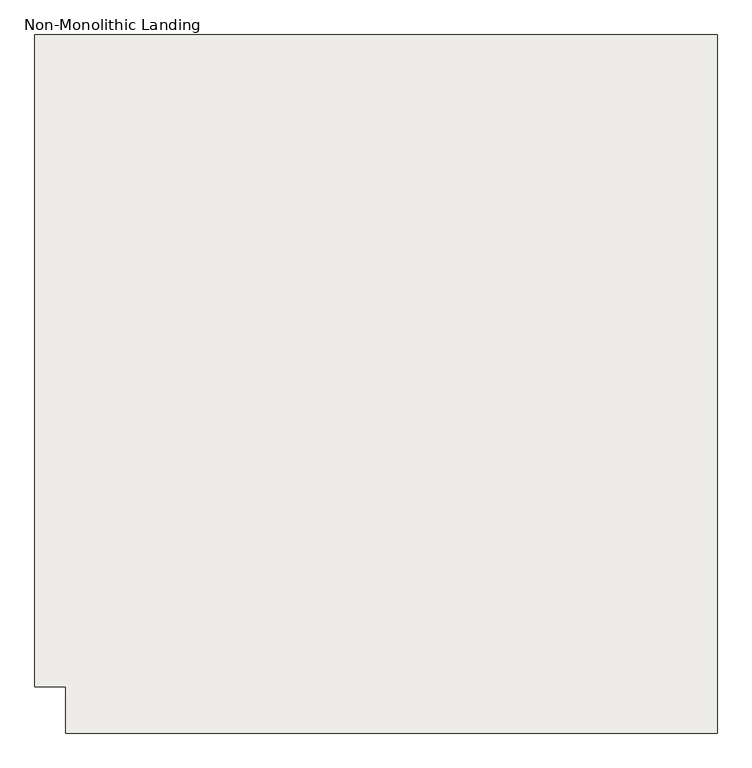
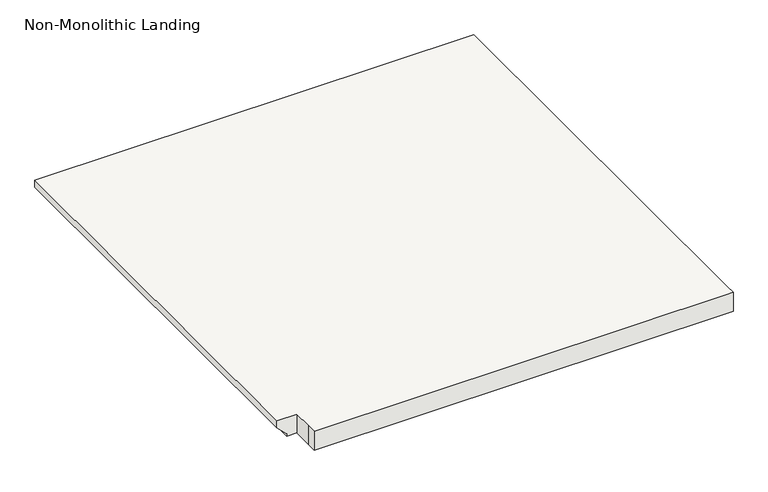
"""IFC4 building model written with IfcOpenShell, lengths in millimetres: slab geometry, Non-Monolithic Landing."""

from ifc_helpers import new_model, si_unit, origin, place, context, project, spatial, faceted_brep, source, transform, mapped, element, save


def non_monolithic_landing_2a78468c(model_context):
    return source(origin(), model_context, "Body", "Brep", [
        faceted_brep([(2334.73354, -1849.1834702, 1657.35), (2334.73354, -1849.1834702, 1676.4), (2334.73354, -782.3834702, 1676.4), (2334.73354, -782.3834702, 1657.35), (2360.13354, -1849.1834702, 1631.95), (2360.13354, -782.3834702, 1631.95), (2385.53354, -1849.1834702, 1676.4), (2385.53354, -1899.9834702, 1676.4), (2385.53354, -1925.3834702, 1676.4), (3452.33354, -1925.3834702, 1676.4), (3452.33354, -1899.9834702, 1676.4), (3452.33354, -782.3834702, 1676.4), (2360.13354, -1849.1834702, 1625.6), (2360.13354, -782.3834702, 1625.6), (3452.33354, -782.3834702, 1625.6), (3452.33354, -1899.9834702, 1625.6), (3452.33354, -1925.3834702, 1625.6), (2385.53354, -1925.3834702, 1625.6), (2385.53354, -1899.9834702, 1625.6), (2385.53354, -1849.1834702, 1625.6)], [[[0, 1, 2, 3]], [[4, 0, 3, 5]], [[6, 7, 8, 9, 10, 11, 2, 1]], [[12, 13, 14, 15, 16, 17, 18, 19]], [[13, 12, 4, 5]], [[6, 1, 0, 4, 12, 19]], [[7, 6, 19, 18]], [[8, 7, 18, 17]], [[9, 8, 17, 16]], [[10, 9, 16, 15]], [[11, 10, 15, 14]], [[2, 11, 14, 13, 5, 3]]]),
    ])


if __name__ == "__main__":
    model = new_model("IFC4")
    model_context = context("Model", 3, world=origin())
    ifc_project = project(units=[si_unit("LENGTHUNIT", "METRE", prefix="MILLI")], contexts=[model_context])
    site = spatial("IfcSite", under=ifc_project)
    building = spatial("IfcBuilding", under=site)
    placement = place(None, origin())
    non_monolithic_landing_shape = non_monolithic_landing_2a78468c(model_context)
    element("IfcSlab", 1, ObjectType="Non-Monolithic Landing", at=placement, inside=building, context=model_context, shape_type="MappedRepresentation", body=[
        mapped(non_monolithic_landing_shape, transform((0.0, 0.0, 0.0), x_axis=(1.0, 0.0, 0.0), y_axis=(0.0, 1.0, 0.0), z_axis=(0.0, 0.0, 1.0))),
    ])
    save(model, "model.ifc")
